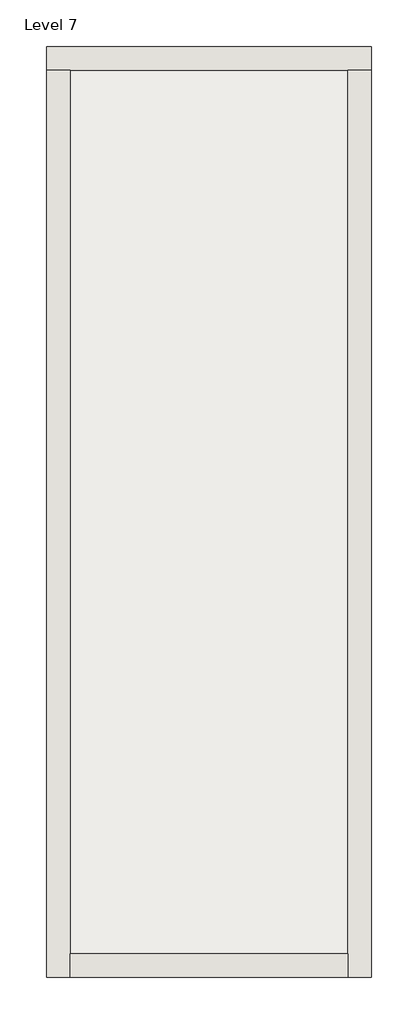
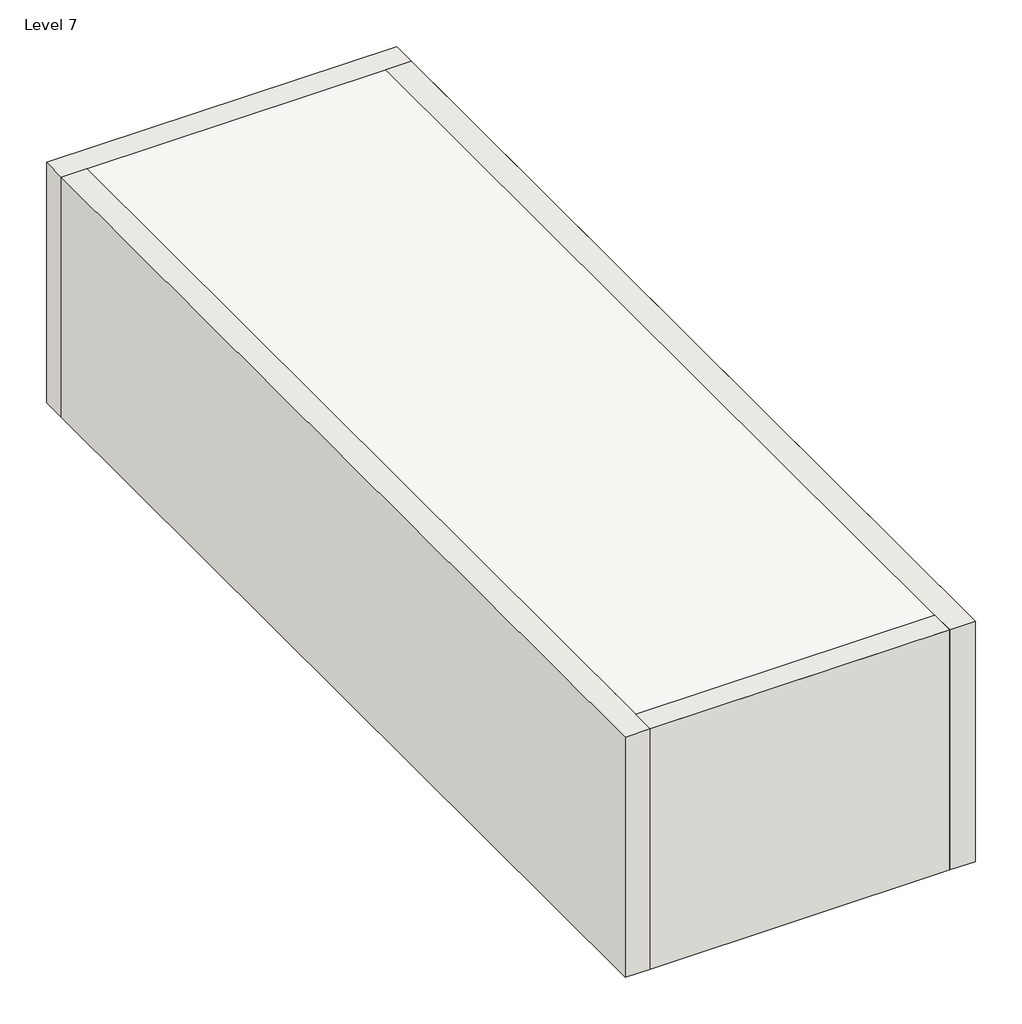
# One storey: 4 walls, 1 slab.
"""IFC4 building model written with IfcOpenShell, lengths in millimetres."""

from ifc_helpers import new_model, si_unit, frame, origin, place, context, project, spatial, polyline, outline, extrude, faceted_brep, element, save

model = new_model("IFC4")

# Units and contexts
model_context = context("Model", 3, world=origin())
ifc_project = project(units=[si_unit("LENGTHUNIT", "METRE", prefix="MILLI")], contexts=[model_context])

# Site, building, storey
site = spatial("IfcSite", under=ifc_project)
building = spatial("IfcBuilding", under=site)
storey = spatial("IfcBuildingStorey", under=building, Name="Level 7", Elevation=15240.0)

# Slab
placement = place(None, origin())
element("IfcSlab", 1, ObjectType="Generic - 12\"", at=placement, inside=storey, context=model_context, shape_type="SweptSolid", body=[
    extrude(outline(polyline([(15.2772392, -109.5466977), (-2905.7230786, -109.5466977), (-2905.7230786, 8907.4533023), (15.2772392, 8907.4533023), (15.2772392, -109.5466977)])), frame((0.0, 0.0, 14173.2170652), z_axis=(0.0, 0.0, 1.0), x_axis=(1.0, 0.0, 0.0)), (0.0, 0.0, 1.0), 304.8),
])

# Walls
element("IfcWall", 2, ObjectType="9\"", at=placement, inside=storey, context=model_context, shape_type="Brep", body=[
    faceted_brep([(-213.3227608, 8678.8533023, 12192.0), (-213.3227608, 119.0533023, 12192.0), (-213.3227608, -109.5466977, 12192.0), (-213.3227608, -109.5466977, 14478.0170652), (-213.3227608, 119.0533023, 14478.0170652), (-213.3227608, 8678.8533023, 14478.0170652), (15.2772392, 8678.8533023, 12192.0), (15.2772392, 8678.8533023, 14478.0170652), (15.2772392, -109.5466977, 14478.0170652), (15.2772392, -109.5466977, 12192.0)], [[[0, 1, 2, 3, 4, 5]], [[6, 7, 8, 9]], [[2, 1, 0, 6, 9]], [[5, 4, 3, 8, 7]], [[0, 5, 7, 6]], [[3, 2, 9, 8]]]),
])
element("IfcWall", 3, ObjectType="9\"", at=placement, inside=storey, context=model_context, shape_type="Brep", body=[
    faceted_brep([(15.2772392, 8907.4533023, 12192.0), (-3134.3230786, 8907.4533023, 12192.0), (-3134.3230786, 8907.4533023, 14478.0170652), (15.2772392, 8907.4533023, 14478.0170652), (15.2772392, 8678.8533023, 12192.0), (15.2772392, 8678.8533023, 14478.0170652), (-213.3227608, 8678.8533023, 14478.0170652), (-2905.7230786, 8678.8533023, 14478.0170652), (-3134.3230786, 8678.8533023, 14478.0170652), (-3134.3230786, 8678.8533023, 12192.0), (-2905.7230786, 8678.8533023, 12192.0), (-213.3227608, 8678.8533023, 12192.0)], [[[0, 1, 2, 3]], [[4, 5, 6, 7, 8, 9, 10, 11]], [[1, 0, 4, 11, 10, 9]], [[3, 2, 8, 7, 6, 5]], [[0, 3, 5, 4]], [[2, 1, 9, 8]]]),
])
element("IfcWall", 4, ObjectType="9\"", at=placement, inside=storey, context=model_context, shape_type="Brep", body=[
    faceted_brep([(-3134.3230786, 8678.8533023, 12192.0), (-3134.3230786, -109.5466977, 12192.0), (-3134.3230786, -109.5466977, 14478.0170652), (-3134.3230786, 8678.8533023, 14478.0170652), (-2905.7230786, 8678.8533023, 12192.0), (-2905.7230786, 8678.8533023, 14478.0170652), (-2905.7230786, 119.0533023, 14478.0170652), (-2905.7230786, -109.5466977, 14478.0170652), (-2905.7230786, -109.5466977, 12192.0), (-2905.7230786, 119.0533023, 12192.0)], [[[0, 1, 2, 3]], [[4, 5, 6, 7, 8, 9]], [[1, 0, 4, 9, 8]], [[3, 2, 7, 6, 5]], [[0, 3, 5, 4]], [[2, 1, 8, 7]]]),
])
element("IfcWall", 5, ObjectType="9\"", at=placement, inside=storey, context=model_context, shape_type="SweptSolid", body=[
    extrude(outline(polyline([(-213.3227608, -109.5466977), (-2905.7230786, -109.5466977), (-2905.7230786, 119.0533023), (-213.3227608, 119.0533023), (-213.3227608, -109.5466977)])), frame((0.0, 0.0, 12192.0), z_axis=(0.0, 0.0, 1.0), x_axis=(1.0, 0.0, 0.0)), (0.0, 0.0, 1.0), 2286.0170652),
])

save(model, "model.ifc")

# Revit data of these elements
# Type "Generic - 12\""
#   Assembly Code = "B1010"
#   Function = 0
#   Layers, outside or top first: 1' - 0" no material (function 1)
# Type "9\""
#   Assembly Code = "B2010"
#   Layers, outside or top first: 0' - 9" no material (function 1)
# Element 1 (IfcSlab, "Generic - 12\"")
#   Height Offset From Level = -2' - 5.99933"
#   Phase Created = New Construction
#   Materials on its faces: "Default Floor", "1 wall"
# Elements 2, 3, 4, 5 (IfcWall, "9\"")
#   built-in parameter 1001111 = -10' - 0"
#   Top Offset = 0' - 0"
#   Base Offset = -10' - 0"
#   Unconnected Height = 7' - 6.00067"
#   wall height = 7' - 6.00067"
#   Phase Created = New Construction
#   Base Constraint = Level 7
#   Materials on its faces: "Default Wall", "1 wall"
# Materials
#   "Default Floor": colour RGB 128 128 128, transparency 0, Cost = 0
#   "1 wall": class "Generic", colour RGB 244 245 241, transparency 0, Cost = 0
#   "Default Wall": colour RGB 128 128 128, transparency 0, Cost = 0
